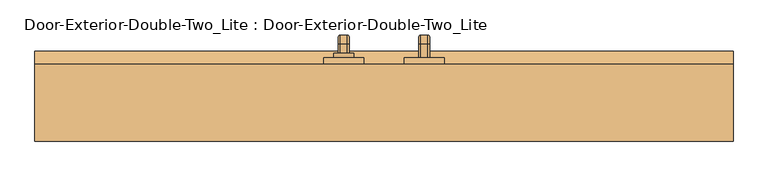
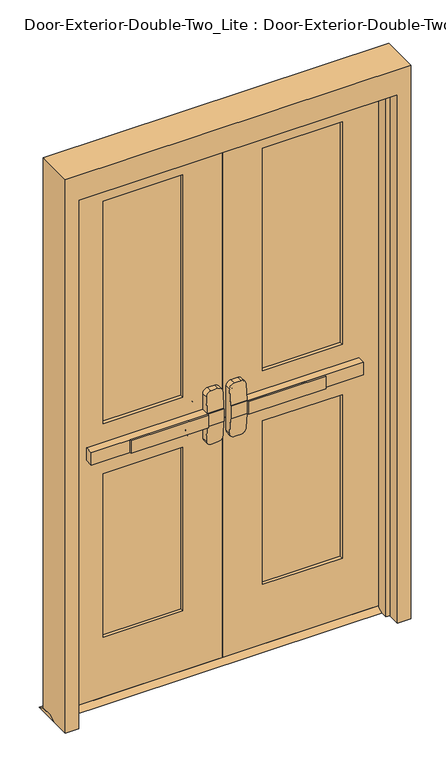
"""IFC4 building model written with IfcOpenShell, lengths in millimetres: door geometry, Door-Exterior-Double-Two_Lite : Door-Exterior-Double-Two_Lite."""

from ifc_helpers import new_model, si_unit, point, frame, frame_2d, origin, place, context, project, spatial, polyline, circle_curve, ellipse_curve, trimmed, segment, composite_curve, outline, extrude, faceted_brep, source, transform, mapped, element, save
from ifc_brep_helpers import plane_surface, cylinder_surface, revolved_surface, advanced_brep


def door_exterior_double_two_lite_door_exterior_double_two_lite_a6b01c7a(model_context):
    return source(origin(), model_context, "Body", "SolidModel", [
        extrude(outline(polyline([(-372.5333333, 12.7), (-372.5333333, 19.05), (-76.2, 19.05), (-76.2, 12.7), (-372.5333333, 12.7)])), frame((0.0, 0.0, 990.6), z_axis=(0.0, 0.0, 1.0), x_axis=(1.0, 0.0, 0.0)), (0.0, 0.0, 1.0), 50.8),
        advanced_brep(
        [(-12.7, 19.05, 1041.4), (-76.2, 19.05, 1041.4), (-520.7, 19.05, 1041.4), (-520.7, 19.05, 990.6), (-76.2, 19.05, 990.6), (-12.7, 19.05, 990.6), (-520.7, 50.8, 1041.4), (-76.2, 50.8, 1041.4), (-76.2, 50.8, 1104.9), (-57.15, 50.8, 1123.95), (-31.75, 50.8, 1123.95), (-12.7, 50.8, 1104.9), (-12.7, 50.8, 927.1), (-31.75, 50.8, 908.05), (-57.15, 50.8, 908.05), (-76.2, 50.8, 927.1), (-76.2, 50.8, 990.6), (-520.7, 50.8, 990.6), (-12.7, 22.2252467, 1041.4), (-76.2, 22.2252467, 1041.4), (-12.7, 22.2252467, 990.6), (-12.7, 27.2354269, 927.1), (-12.7, 27.2354269, 1104.9), (-76.2, 22.2252467, 990.6), (-76.2, 27.2354269, 1104.9), (-76.2, 27.2354269, 927.1), (-57.15, 28.738481, 1123.95), (-31.75, 28.738481, 1123.95), (-31.75, 28.738481, 908.05), (-57.15, 28.738481, 908.05)],
        [
            (0, 1),
            (1, 2),
            (2, 3),
            (3, 4),
            (4, 5),
            (5, 0),
            (6, 7),
            (7, 8),
            (8, 9, circle_curve(frame((-57.15, 50.8, 1104.9), z_axis=(0.0, 1.0, 0.0), x_axis=(-1.0, 0.0, 0.0)), 19.05)),
            (9, 10),
            (10, 11, circle_curve(frame((-31.75, 50.8, 1104.9), z_axis=(0.0, 1.0, 0.0), x_axis=(-1.0, 0.0, 0.0)), 19.05)),
            (11, 12),
            (12, 13, circle_curve(frame((-31.75, 50.8, 927.1), z_axis=(0.0, 1.0, 0.0), x_axis=(-1.0, 0.0, 0.0)), 19.05)),
            (13, 14),
            (14, 15, circle_curve(frame((-57.15, 50.8, 927.1), z_axis=(0.0, 1.0, 0.0), x_axis=(-1.0, 0.0, 0.0)), 19.05)),
            (15, 16),
            (16, 17),
            (17, 6),
            (0, 18),
            (18, 19),
            (19, 7),
            (6, 2),
            (5, 20),
            (20, 21),
            (21, 12),
            (11, 22),
            (22, 18),
            (16, 23),
            (23, 20),
            (3, 17),
            (19, 24),
            (24, 8),
            (15, 25),
            (25, 23),
            (9, 26),
            (26, 27),
            (27, 10),
            (13, 28),
            (28, 29),
            (29, 14),
            (29, 25, ellipse_curve(frame((-57.15, 27.2354269, 927.1), z_axis=(0.0, 0.9969018152893365, 0.07865602756830282), x_axis=(0.0, -0.07865602756830208, 0.9969018152893365)), 19.1092038, 19.05)),
            (24, 26, ellipse_curve(frame((-57.15, 27.2354269, 1104.9), z_axis=(0.0, 0.9969018152893376, -0.07865602756828934), x_axis=(0.0, -0.078656027568288, -0.9969018152893377)), 19.1092038, 19.05)),
            (27, 22, ellipse_curve(frame((-31.75, 27.2354269, 1104.9), z_axis=(0.0, 0.9969018152893376, -0.07865602756828934), x_axis=(0.0, -0.078656027568288, -0.9969018152893377)), 19.1092038, 19.05)),
            (21, 28, ellipse_curve(frame((-31.75, 27.2354269, 927.1), z_axis=(0.0, 0.9969018152893365, 0.07865602756830282), x_axis=(0.0, -0.07865602756830208, 0.9969018152893365)), 19.1092038, 19.05)),
        ],
        [
            plane_surface(frame((-12.7, 19.05, 1041.4), z_axis=(0.0, -1.0, 0.0), x_axis=(1.0, 0.0, 0.0))),
            plane_surface(frame((-12.7, 50.8, 1041.4), z_axis=(0.0, 1.0, 0.0), x_axis=(-1.0, 0.0, 0.0))),
            plane_surface(frame((-520.7, 19.05, 1041.4), z_axis=(0.0, 0.0, 1.0), x_axis=(0.0, 1.0, 0.0))),
            plane_surface(frame((-12.7, 19.05, 1041.4), z_axis=(1.0, 0.0, 0.0), x_axis=(0.0, 1.0, 0.0))),
            plane_surface(frame((-12.7, 19.05, 990.6), z_axis=(0.0, 0.0, -1.0), x_axis=(0.0, 1.0, 0.0))),
            plane_surface(frame((-520.7, 19.05, 990.6), z_axis=(-1.0, 0.0, 0.0), x_axis=(0.0, 1.0, 0.0))),
            plane_surface(frame((-76.2, 22.2252467, 927.1), z_axis=(-1.0, 0.0, 0.0), x_axis=(0.0, 1.0, 0.0))),
            plane_surface(frame((-57.15, 22.2252467, 1123.95), z_axis=(0.0, 0.0, 1.0), x_axis=(0.0, 1.0, 0.0))),
            plane_surface(frame((-31.75, 22.2252467, 908.05), z_axis=(0.0, 0.0, -1.0), x_axis=(0.0, 1.0, 0.0))),
            cylinder_surface(frame((-57.15, 50.8, 927.1), z_axis=(0.0, -1.0, 0.0), x_axis=(-1.0, 0.0, 0.0)), 19.05),
            cylinder_surface(frame((-57.15, 50.8, 1104.9), z_axis=(0.0, -1.0, 0.0), x_axis=(-1.0, 0.0, 0.0)), 19.05),
            cylinder_surface(frame((-31.75, 50.8, 1104.9), z_axis=(0.0, -1.0, 0.0), x_axis=(-1.0, 0.0, 0.0)), 19.05),
            cylinder_surface(frame((-31.75, 50.8, 927.1), z_axis=(0.0, -1.0, 0.0), x_axis=(-1.0, 0.0, 0.0)), 19.05),
            plane_surface(frame((-76.2, 22.2252467, 1041.4), z_axis=(0.0, -0.9969018152893376, 0.07865602756828934), x_axis=(1.0, 0.0, 0.0))),
            plane_surface(frame((-76.2, 28.738481, 908.05), z_axis=(0.0, -0.9969018152893365, -0.07865602756830282), x_axis=(1.0, 0.0, 0.0))),
        ],
        [
            (0, [[1, 2, 3, 4, 5, 6]]),
            (1, [[7, 8, 9, 10, 11, 12, 13, 14, 15, 16, 17, 18]]),
            (2, [[-2, -1, 19, 20, 21, -7, 22]]),
            (3, [[23, 24, 25, -12, 26, 27, -19, -6]]),
            (4, [[-17, 28, 29, -23, -5, -4, 30]]),
            (5, [[-22, -18, -30, -3]]),
            (6, [[-21, 31, 32, -8]]),
            (6, [[33, 34, -28, -16]]),
            (7, [[35, 36, 37, -10]]),
            (8, [[38, 39, 40, -14]]),
            (9, [[-40, 41, -33, -15]]),
            (10, [[-32, 42, -35, -9]]),
            (11, [[-37, 43, -26, -11]]),
            (12, [[-25, 44, -38, -13]]),
            (13, [[-27, -43, -36, -42, -31, -20]]),
            (14, [[-29, -34, -41, -39, -44, -24]]),
        ],
    ),
        extrude(outline(polyline([(95.25, 12.7), (120.65, 0.0), (25.4, 0.0), (50.8, 12.7), (95.25, 12.7)])), frame((-660.4, 0.0, 0.0), z_axis=(1.0, 0.0, 0.0), x_axis=(0.0, 1.0, 0.0)), (0.0, 0.0, 1.0), 1320.8),
        extrude(outline(polyline([(372.5333333, 12.7), (76.2, 12.7), (76.2, 19.05), (372.5333333, 19.05), (372.5333333, 12.7)])), frame((0.0, 0.0, 990.6), z_axis=(0.0, 0.0, 1.0), x_axis=(1.0, 0.0, 0.0)), (0.0, 0.0, 1.0), 50.8),
        advanced_brep(
        [(12.7, 19.05, 1041.4), (12.7, 19.05, 990.6), (76.2, 19.05, 990.6), (520.7, 19.05, 990.6), (520.7, 19.05, 1041.4), (76.2, 19.05, 1041.4), (520.7, 50.8, 1041.4), (520.7, 50.8, 990.6), (76.2, 50.8, 990.6), (76.2, 50.8, 927.1), (57.15, 50.8, 908.05), (31.75, 50.8, 908.05), (12.7, 50.8, 927.1), (12.7, 50.8, 1104.9), (31.75, 50.8, 1123.95), (57.15, 50.8, 1123.95), (76.2, 50.8, 1104.9), (76.2, 50.8, 1041.4), (76.2, 22.2252467, 1041.4), (12.7, 22.2252467, 1041.4), (12.7, 27.2354269, 1104.9), (12.7, 27.2354269, 927.1), (12.7, 22.2252467, 990.6), (76.2, 22.2252467, 990.6), (76.2, 27.2354269, 927.1), (76.2, 27.2354269, 1104.9), (31.75, 28.738481, 1123.95), (57.15, 28.738481, 1123.95), (57.15, 28.738481, 908.05), (31.75, 28.738481, 908.05)],
        [
            (0, 1),
            (1, 2),
            (2, 3),
            (3, 4),
            (4, 5),
            (5, 0),
            (6, 7),
            (7, 8),
            (8, 9),
            (9, 10, circle_curve(frame((57.15, 50.8, 927.1), z_axis=(0.0, 1.0, 0.0), x_axis=(1.0, 0.0, 0.0)), 19.05)),
            (10, 11),
            (11, 12, circle_curve(frame((31.75, 50.8, 927.1), z_axis=(0.0, 1.0, 0.0), x_axis=(1.0, 0.0, 0.0)), 19.05)),
            (12, 13),
            (13, 14, circle_curve(frame((31.75, 50.8, 1104.9), z_axis=(0.0, 1.0, 0.0), x_axis=(1.0, 0.0, 0.0)), 19.05)),
            (14, 15),
            (15, 16, circle_curve(frame((57.15, 50.8, 1104.9), z_axis=(0.0, 1.0, 0.0), x_axis=(1.0, 0.0, 0.0)), 19.05)),
            (16, 17),
            (17, 6),
            (4, 6),
            (17, 18),
            (18, 19),
            (19, 0),
            (19, 20),
            (20, 13),
            (12, 21),
            (21, 22),
            (22, 1),
            (7, 3),
            (22, 23),
            (23, 8),
            (23, 24),
            (24, 9),
            (16, 25),
            (25, 18),
            (14, 26),
            (26, 27),
            (27, 15),
            (10, 28),
            (28, 29),
            (29, 11),
            (24, 28, ellipse_curve(frame((57.15, 27.2354269, 927.1), z_axis=(0.0, 0.9969018152893365, 0.07865602756830282), x_axis=(0.0, -0.07865602756830208, 0.9969018152893365)), 19.1092038, 19.05)),
            (27, 25, ellipse_curve(frame((57.15, 27.2354269, 1104.9), z_axis=(0.0, 0.9969018152893376, -0.07865602756828934), x_axis=(0.0, -0.078656027568288, -0.9969018152893377)), 19.1092038, 19.05)),
            (20, 26, ellipse_curve(frame((31.75, 27.2354269, 1104.9), z_axis=(0.0, 0.9969018152893376, -0.07865602756828934), x_axis=(0.0, -0.078656027568288, -0.9969018152893377)), 19.1092038, 19.05)),
            (29, 21, ellipse_curve(frame((31.75, 27.2354269, 927.1), z_axis=(0.0, 0.9969018152893365, 0.07865602756830282), x_axis=(0.0, -0.07865602756830208, 0.9969018152893365)), 19.1092038, 19.05)),
        ],
        [
            plane_surface(frame((12.7, 19.05, 1041.4), z_axis=(0.0, -1.0, 0.0), x_axis=(-1.0, 0.0, 0.0))),
            plane_surface(frame((12.7, 50.8, 1041.4), z_axis=(0.0, 1.0, 0.0), x_axis=(1.0, 0.0, 0.0))),
            plane_surface(frame((520.7, 19.05, 1041.4), z_axis=(0.0, 0.0, 1.0), x_axis=(0.0, 1.0, 0.0))),
            plane_surface(frame((12.7, 19.05, 1041.4), z_axis=(-1.0, 0.0, 0.0), x_axis=(0.0, 1.0, 0.0))),
            plane_surface(frame((12.7, 19.05, 990.6), z_axis=(0.0, 0.0, -1.0), x_axis=(0.0, 1.0, 0.0))),
            plane_surface(frame((520.7, 19.05, 990.6), z_axis=(1.0, 0.0, 0.0), x_axis=(0.0, 1.0, 0.0))),
            plane_surface(frame((76.2, 22.2252467, 927.1), z_axis=(1.0, 0.0, 0.0), x_axis=(0.0, 1.0, 0.0))),
            plane_surface(frame((57.15, 22.2252467, 1123.95), z_axis=(0.0, 0.0, 1.0), x_axis=(0.0, 1.0, 0.0))),
            plane_surface(frame((31.75, 22.2252467, 908.05), z_axis=(0.0, 0.0, -1.0), x_axis=(0.0, 1.0, 0.0))),
            cylinder_surface(frame((57.15, 50.8, 927.1), z_axis=(0.0, -1.0, 0.0), x_axis=(1.0, 0.0, 0.0)), 19.05),
            cylinder_surface(frame((57.15, 50.8, 1104.9), z_axis=(0.0, -1.0, 0.0), x_axis=(1.0, 0.0, 0.0)), 19.05),
            cylinder_surface(frame((31.75, 50.8, 1104.9), z_axis=(0.0, -1.0, 0.0), x_axis=(1.0, 0.0, 0.0)), 19.05),
            cylinder_surface(frame((31.75, 50.8, 927.1), z_axis=(0.0, -1.0, 0.0), x_axis=(1.0, 0.0, 0.0)), 19.05),
            plane_surface(frame((76.2, 22.2252467, 1041.4), z_axis=(0.0, -0.9969018152893376, 0.07865602756828934), x_axis=(-1.0, 0.0, 0.0))),
            plane_surface(frame((76.2, 28.738481, 908.05), z_axis=(0.0, -0.9969018152893365, -0.07865602756830282), x_axis=(-1.0, 0.0, 0.0))),
        ],
        [
            (0, [[1, 2, 3, 4, 5, 6]]),
            (1, [[7, 8, 9, 10, 11, 12, 13, 14, 15, 16, 17, 18]]),
            (2, [[19, -18, 20, 21, 22, -6, -5]]),
            (3, [[-1, -22, 23, 24, -13, 25, 26, 27]]),
            (4, [[28, -3, -2, -27, 29, 30, -8]]),
            (5, [[-4, -28, -7, -19]]),
            (6, [[-9, -30, 31, 32]]),
            (6, [[-17, 33, 34, -20]]),
            (7, [[-15, 35, 36, 37]]),
            (8, [[-11, 38, 39, 40]]),
            (9, [[-10, -32, 41, -38]]),
            (10, [[-16, -37, 42, -33]]),
            (11, [[-14, -24, 43, -35]]),
            (12, [[-12, -40, 44, -25]]),
            (13, [[-21, -34, -42, -36, -43, -23]]),
            (14, [[-26, -44, -39, -41, -31, -29]]),
        ],
    ),
        advanced_brep(
        [(66.2, 107.95, 1017.190625), (66.2, 107.95, 1014.809375), (69.771875, 107.95, 1011.2375), (82.6284594, 107.95, 1011.2375), (86.2, 107.95, 1014.8090406), (86.2, 107.95, 1017.190625), (82.628125, 107.95, 1020.7625), (69.771875, 107.95, 1020.7625), (66.2, 107.95, 887.809375), (69.771875, 107.95, 884.2375), (82.628125, 107.95, 884.2375), (86.2, 107.95, 887.809375), (86.2, 107.95, 890.1909594), (82.6284594, 107.95, 893.7625), (69.771875, 107.95, 893.7625), (66.2, 107.95, 890.190625), (66.2, 133.35, 1017.190625), (66.2, 147.240625, 1003.3), (66.2, 147.240625, 901.7), (66.2, 133.35, 887.809375), (66.2, 133.35, 890.190625), (66.2, 144.859375, 901.7), (66.2, 144.859375, 1003.3), (66.2, 133.35, 1014.809375), (69.771875, 133.35, 1011.2375), (82.6284594, 133.35, 1011.2375), (86.2, 133.35, 1014.8090406), (86.2, 144.8590406, 1003.3), (86.2, 144.8590406, 901.7), (86.2, 133.35, 890.1909594), (86.2, 133.35, 887.809375), (86.2, 147.240625, 901.7), (86.2, 147.240625, 1003.3), (86.2, 133.35, 1017.190625), (82.628125, 133.35, 1020.7625), (69.771875, 133.35, 1020.7625), (69.771875, 141.2875, 1003.3), (82.6284594, 141.2875, 1003.3), (82.628125, 150.8125, 1003.3), (69.771875, 150.8125, 1003.3), (69.771875, 141.2875, 901.7), (82.6284594, 141.2875, 901.7), (82.628125, 150.8125, 901.7), (69.771875, 150.8125, 901.7), (69.771875, 133.35, 893.7625), (82.6284594, 133.35, 893.7625), (82.628125, 133.35, 884.2375), (69.771875, 133.35, 884.2375)],
        [
            (0, 1),
            (1, 2, circle_curve(frame((69.771875, 107.95, 1014.809375), z_axis=(0.0, -1.0, 0.0), x_axis=(0.0, 0.0, 1.0)), 3.571875)),
            (2, 3),
            (3, 4, circle_curve(frame((82.6284594, 107.95, 1014.8090406), z_axis=(0.0, -1.0, 0.0), x_axis=(0.0, 0.0, 1.0)), 3.5715406)),
            (4, 5),
            (5, 6, circle_curve(frame((82.628125, 107.95, 1017.190625), z_axis=(0.0, -1.0, 0.0), x_axis=(0.0, 0.0, 1.0)), 3.571875)),
            (6, 7),
            (7, 0, circle_curve(frame((69.771875, 107.95, 1017.190625), z_axis=(0.0, -1.0, 0.0), x_axis=(0.0, 0.0, 1.0)), 3.571875)),
            (8, 9, circle_curve(frame((69.771875, 107.95, 887.809375), z_axis=(0.0, -1.0, 0.0), x_axis=(0.0, 0.0, -1.0)), 3.571875)),
            (9, 10),
            (10, 11, circle_curve(frame((82.628125, 107.95, 887.809375), z_axis=(0.0, -1.0, 0.0), x_axis=(0.0, 0.0, -1.0)), 3.571875)),
            (11, 12),
            (12, 13, circle_curve(frame((82.6284594, 107.95, 890.1909594), z_axis=(0.0, -1.0, 0.0), x_axis=(0.0, 0.0, -1.0)), 3.5715406)),
            (13, 14),
            (14, 15, circle_curve(frame((69.771875, 107.95, 890.190625), z_axis=(0.0, -1.0, 0.0), x_axis=(0.0, 0.0, -1.0)), 3.571875)),
            (15, 8),
            (0, 16),
            (16, 17, circle_curve(frame((66.2, 133.35, 1003.3), z_axis=(-1.0, 0.0, 0.0), x_axis=(0.0, 0.0, 1.0)), 13.890625)),
            (17, 18),
            (18, 19, circle_curve(frame((66.2, 133.35, 901.7), z_axis=(-1.0, 0.0, 0.0), x_axis=(0.0, 1.0, 0.0)), 13.890625)),
            (19, 8),
            (15, 20),
            (20, 21, circle_curve(frame((66.2, 133.35, 901.7), z_axis=(1.0, 0.0, 0.0), x_axis=(0.0, 1.0, 0.0)), 11.509375)),
            (21, 22),
            (22, 23, circle_curve(frame((66.2, 133.35, 1003.3), z_axis=(1.0, 0.0, 0.0), x_axis=(0.0, 0.0, 1.0)), 11.509375)),
            (23, 1),
            (23, 24, circle_curve(frame((69.771875, 133.35, 1014.809375), z_axis=(0.0, -1.0, 0.0), x_axis=(0.0, 0.0, 1.0)), 3.571875)),
            (24, 2),
            (24, 25),
            (25, 3),
            (25, 26, circle_curve(frame((82.6284594, 133.35, 1014.8090406), z_axis=(0.0, -1.0, 0.0), x_axis=(0.0, 0.0, 1.0)), 3.5715406)),
            (26, 4),
            (26, 27, circle_curve(frame((86.2, 133.35, 1003.3), z_axis=(-1.0, 0.0, 0.0), x_axis=(0.0, 0.0, 1.0)), 11.5090406)),
            (27, 28),
            (28, 29, circle_curve(frame((86.2, 133.35, 901.7), z_axis=(-1.0, 0.0, 0.0), x_axis=(0.0, 1.0, 0.0)), 11.5090406)),
            (29, 12),
            (11, 30),
            (30, 31, circle_curve(frame((86.2, 133.35, 901.7), z_axis=(1.0, 0.0, 0.0), x_axis=(0.0, 1.0, 0.0)), 13.890625)),
            (31, 32),
            (32, 33, circle_curve(frame((86.2, 133.35, 1003.3), z_axis=(1.0, 0.0, 0.0), x_axis=(0.0, 0.0, 1.0)), 13.890625)),
            (33, 5),
            (33, 34, circle_curve(frame((82.628125, 133.35, 1017.190625), z_axis=(0.0, -1.0, 0.0), x_axis=(0.0, 0.0, 1.0)), 3.571875)),
            (34, 6),
            (34, 35),
            (35, 7),
            (35, 16, circle_curve(frame((69.771875, 133.35, 1017.190625), z_axis=(0.0, -1.0, 0.0), x_axis=(0.0, 0.0, 1.0)), 3.571875)),
            (36, 24, circle_curve(frame((69.771875, 133.35, 1003.3), z_axis=(1.0, 0.0, 0.0), x_axis=(0.0, 0.0, 1.0)), 7.9375)),
            (22, 36, circle_curve(frame((69.771875, 144.859375, 1003.3), z_axis=(0.0, 0.0, 1.0), x_axis=(0.0, 1.0, 0.0)), 3.571875)),
            (37, 25, circle_curve(frame((82.6284594, 133.35, 1003.3), z_axis=(1.0, 0.0, 0.0), x_axis=(0.0, 0.0, 1.0)), 7.9375)),
            (36, 37),
            (37, 27, circle_curve(frame((82.6284594, 144.8590406, 1003.3), z_axis=(0.0, 0.0, 1.0), x_axis=(0.0, 1.0, 0.0)), 3.5715406)),
            (38, 34, circle_curve(frame((82.628125, 133.35, 1003.3), z_axis=(1.0, 0.0, 0.0), x_axis=(0.0, 0.0, 1.0)), 17.4625)),
            (32, 38, circle_curve(frame((82.628125, 147.240625, 1003.3), z_axis=(0.0, 0.0, 1.0), x_axis=(0.0, 1.0, 0.0)), 3.571875)),
            (39, 35, circle_curve(frame((69.771875, 133.35, 1003.3), z_axis=(1.0, 0.0, 0.0), x_axis=(0.0, 0.0, 1.0)), 17.4625)),
            (38, 39),
            (39, 17, circle_curve(frame((69.771875, 147.240625, 1003.3), z_axis=(0.0, 0.0, 1.0), x_axis=(0.0, 1.0, 0.0)), 3.571875)),
            (21, 40, circle_curve(frame((69.771875, 144.859375, 901.7), z_axis=(0.0, 0.0, 1.0), x_axis=(0.0, 1.0, 0.0)), 3.571875)),
            (40, 36),
            (40, 41),
            (41, 37),
            (41, 28, circle_curve(frame((82.6284594, 144.8590406, 901.7), z_axis=(0.0, 0.0, 1.0), x_axis=(0.0, 1.0, 0.0)), 3.5715406)),
            (31, 42, circle_curve(frame((82.628125, 147.240625, 901.7), z_axis=(0.0, 0.0, 1.0), x_axis=(0.0, 1.0, 0.0)), 3.571875)),
            (42, 38),
            (42, 43),
            (43, 39),
            (43, 18, circle_curve(frame((69.771875, 147.240625, 901.7), z_axis=(0.0, 0.0, 1.0), x_axis=(0.0, 1.0, 0.0)), 3.571875)),
            (44, 40, circle_curve(frame((69.771875, 133.35, 901.7), z_axis=(1.0, 0.0, 0.0), x_axis=(0.0, 1.0, 0.0)), 7.9375)),
            (20, 44, circle_curve(frame((69.771875, 133.35, 890.190625), z_axis=(0.0, 1.0, 0.0), x_axis=(0.0, 0.0, -1.0)), 3.571875)),
            (45, 41, circle_curve(frame((82.6284594, 133.35, 901.7), z_axis=(1.0, 0.0, 0.0), x_axis=(0.0, 1.0, 0.0)), 7.9375)),
            (44, 45),
            (45, 29, circle_curve(frame((82.6284594, 133.35, 890.1909594), z_axis=(0.0, 1.0, 0.0), x_axis=(0.0, 0.0, -1.0)), 3.5715406)),
            (46, 42, circle_curve(frame((82.628125, 133.35, 901.7), z_axis=(1.0, 0.0, 0.0), x_axis=(0.0, 1.0, 0.0)), 17.4625)),
            (30, 46, circle_curve(frame((82.628125, 133.35, 887.809375), z_axis=(0.0, 1.0, 0.0), x_axis=(0.0, 0.0, -1.0)), 3.571875)),
            (47, 43, circle_curve(frame((69.771875, 133.35, 901.7), z_axis=(1.0, 0.0, 0.0), x_axis=(0.0, 1.0, 0.0)), 17.4625)),
            (46, 47),
            (47, 19, circle_curve(frame((69.771875, 133.35, 887.809375), z_axis=(0.0, 1.0, 0.0), x_axis=(0.0, 0.0, -1.0)), 3.571875)),
            (14, 44),
            (13, 45),
            (10, 46),
            (9, 47),
        ],
        [
            plane_surface(frame((76.2, 107.95, 1016.0), z_axis=(0.0, -1.0, 0.0), x_axis=(1.0, 0.0, 0.0))),
            plane_surface(frame((76.2, 107.95, 889.0), z_axis=(0.0, -1.0, 0.0), x_axis=(1.0, 0.0, 0.0))),
            plane_surface(frame((66.2, 107.95, 1017.190625), z_axis=(-1.0, 0.0, 0.0), x_axis=(0.0, 1.0, 0.0))),
            cylinder_surface(frame((69.771875, 107.95, 1014.809375), z_axis=(0.0, -1.0, 0.0), x_axis=(0.0, 0.0, 1.0)), 3.571875),
            plane_surface(frame((69.771875, 107.95, 1011.2375), z_axis=(0.0, 0.0, -1.0), x_axis=(0.0, 1.0, 0.0))),
            cylinder_surface(frame((82.6284594, 107.95, 1014.8090406), z_axis=(0.0, -1.0, 0.0), x_axis=(0.0, 0.0, 1.0)), 3.5715406),
            plane_surface(frame((86.2, 107.95, 1014.8090406), z_axis=(1.0, 0.0, 0.0), x_axis=(0.0, 1.0, 0.0))),
            cylinder_surface(frame((82.628125, 107.95, 1017.190625), z_axis=(0.0, -1.0, 0.0), x_axis=(0.0, 0.0, 1.0)), 3.571875),
            plane_surface(frame((82.628125, 107.95, 1020.7625), z_axis=(0.0, 0.0, 1.0), x_axis=(0.0, 1.0, 0.0))),
            cylinder_surface(frame((69.771875, 107.95, 1017.190625), z_axis=(0.0, -1.0, 0.0), x_axis=(0.0, 0.0, 1.0)), 3.571875),
            revolved_surface(trimmed(ellipse_curve(frame((69.771875, 133.35, 1014.809375), z_axis=(0.0, -1.0, 0.0), x_axis=(0.0, 0.0, 1.0)), 3.571875, 3.571875), [point((66.2, 133.35, 1014.809375))], [point((69.771875, 133.35, 1011.2375))], True, "CARTESIAN"), (76.2, 133.35, 1003.3), (-1.0, 0.0, 0.0)),
            revolved_surface(polyline([(69.771875, 133.35, 1011.2375), (82.6284594, 133.35, 1011.2375)]), (76.2, 133.35, 1003.3), (-1.0, 0.0, 0.0)),
            revolved_surface(trimmed(ellipse_curve(frame((82.6284594, 133.35, 1014.8090406), z_axis=(0.0, -1.0, 0.0), x_axis=(0.0, 0.0, 1.0)), 3.5715406, 3.5715406), [point((82.6284594, 133.35, 1011.2375))], [point((86.2, 133.35, 1014.8090406))], True, "CARTESIAN"), (76.2, 133.35, 1003.3), (-1.0, 0.0, 0.0)),
            revolved_surface(trimmed(ellipse_curve(frame((82.628125, 133.35, 1017.190625), z_axis=(0.0, -1.0, 0.0), x_axis=(0.0, 0.0, 1.0)), 3.571875, 3.571875), [point((86.2, 133.35, 1017.190625))], [point((82.628125, 133.35, 1020.7625))], True, "CARTESIAN"), (76.2, 133.35, 1003.3), (-1.0, 0.0, 0.0)),
            cylinder_surface(frame((76.2, 133.35, 1003.3), z_axis=(-1.0, 0.0, 0.0), x_axis=(0.0, 0.0, 1.0)), 17.4625),
            revolved_surface(trimmed(ellipse_curve(frame((69.771875, 133.35, 1017.190625), z_axis=(0.0, -1.0, 0.0), x_axis=(0.0, 0.0, 1.0)), 3.571875, 3.571875), [point((69.771875, 133.35, 1020.7625))], [point((66.2, 133.35, 1017.190625))], True, "CARTESIAN"), (76.2, 133.35, 1003.3), (-1.0, 0.0, 0.0)),
            cylinder_surface(frame((69.771875, 144.859375, 1003.3), z_axis=(0.0, 0.0, 1.0), x_axis=(0.0, 1.0, 0.0)), 3.571875),
            plane_surface(frame((69.771875, 141.2875, 1003.3), z_axis=(0.0, -1.0, 0.0), x_axis=(0.0, 0.0, -1.0))),
            cylinder_surface(frame((82.6284594, 144.8590406, 1003.3), z_axis=(0.0, 0.0, 1.0), x_axis=(0.0, 1.0, 0.0)), 3.5715406),
            cylinder_surface(frame((82.628125, 147.240625, 1003.3), z_axis=(0.0, 0.0, 1.0), x_axis=(0.0, 1.0, 0.0)), 3.571875),
            plane_surface(frame((82.628125, 150.8125, 1003.3), z_axis=(0.0, 1.0, 0.0), x_axis=(0.0, 0.0, -1.0))),
            cylinder_surface(frame((69.771875, 147.240625, 1003.3), z_axis=(0.0, 0.0, 1.0), x_axis=(0.0, 1.0, 0.0)), 3.571875),
            revolved_surface(trimmed(ellipse_curve(frame((69.771875, 144.859375, 901.7), z_axis=(0.0, 0.0, 1.0), x_axis=(0.0, 1.0, 0.0)), 3.571875, 3.571875), [point((66.2, 144.859375, 901.7))], [point((69.771875, 141.2875, 901.7))], True, "CARTESIAN"), (76.2, 133.35, 901.7), (-1.0, 0.0, 0.0)),
            revolved_surface(polyline([(69.771875, 141.2875, 901.7), (82.6284594, 141.2875, 901.7)]), (76.2, 133.35, 901.7), (-1.0, 0.0, 0.0)),
            revolved_surface(trimmed(ellipse_curve(frame((82.6284594, 144.8590406, 901.7), z_axis=(0.0, 0.0, 1.0), x_axis=(0.0, 1.0, 0.0)), 3.5715406, 3.5715406), [point((82.6284594, 141.2875, 901.7))], [point((86.2, 144.8590406, 901.7))], True, "CARTESIAN"), (76.2, 133.35, 901.7), (-1.0, 0.0, 0.0)),
            revolved_surface(trimmed(ellipse_curve(frame((82.628125, 147.240625, 901.7), z_axis=(0.0, 0.0, 1.0), x_axis=(0.0, 1.0, 0.0)), 3.571875, 3.571875), [point((86.2, 147.240625, 901.7))], [point((82.628125, 150.8125, 901.7))], True, "CARTESIAN"), (76.2, 133.35, 901.7), (-1.0, 0.0, 0.0)),
            cylinder_surface(frame((76.2, 133.35, 901.7), z_axis=(-1.0, 0.0, 0.0), x_axis=(0.0, 1.0, 0.0)), 17.4625),
            revolved_surface(trimmed(ellipse_curve(frame((69.771875, 147.240625, 901.7), z_axis=(0.0, 0.0, 1.0), x_axis=(0.0, 1.0, 0.0)), 3.571875, 3.571875), [point((69.771875, 150.8125, 901.7))], [point((66.2, 147.240625, 901.7))], True, "CARTESIAN"), (76.2, 133.35, 901.7), (-1.0, 0.0, 0.0)),
            cylinder_surface(frame((69.771875, 133.35, 890.190625), z_axis=(0.0, 1.0, 0.0), x_axis=(0.0, 0.0, -1.0)), 3.571875),
            plane_surface(frame((69.771875, 133.35, 893.7625), z_axis=(0.0, 0.0, 1.0), x_axis=(0.0, -1.0, 0.0))),
            cylinder_surface(frame((82.6284594, 133.35, 890.1909594), z_axis=(0.0, 1.0, 0.0), x_axis=(0.0, 0.0, -1.0)), 3.5715406),
            cylinder_surface(frame((82.628125, 133.35, 887.809375), z_axis=(0.0, 1.0, 0.0), x_axis=(0.0, 0.0, -1.0)), 3.571875),
            plane_surface(frame((82.628125, 133.35, 884.2375), z_axis=(0.0, 0.0, -1.0), x_axis=(0.0, -1.0, 0.0))),
            cylinder_surface(frame((69.771875, 133.35, 887.809375), z_axis=(0.0, 1.0, 0.0), x_axis=(0.0, 0.0, -1.0)), 3.571875),
        ],
        [
            (0, [[1, 2, 3, 4, 5, 6, 7, 8]]),
            (1, [[9, 10, 11, 12, 13, 14, 15, 16]]),
            (2, [[-1, 17, 18, 19, 20, 21, -16, 22, 23, 24, 25, 26]]),
            (3, [[-2, -26, 27, 28]]),
            (4, [[-3, -28, 29, 30]]),
            (5, [[-4, -30, 31, 32]]),
            (6, [[-5, -32, 33, 34, 35, 36, -12, 37, 38, 39, 40, 41]]),
            (7, [[-6, -41, 42, 43]]),
            (8, [[-7, -43, 44, 45]]),
            (9, [[-8, -45, 46, -17]]),
            (10, [[47, -27, -25, 48]]),
            (11, [[49, -29, -47, 50]]),
            (12, [[-33, -31, -49, 51]]),
            (13, [[52, -42, -40, 53]]),
            (14, [[54, -44, -52, 55]]),
            (15, [[-18, -46, -54, 56]]),
            (16, [[-48, -24, 57, 58]]),
            (17, [[-50, -58, 59, 60]]),
            (18, [[-51, -60, 61, -34]]),
            (19, [[-53, -39, 62, 63]]),
            (20, [[-55, -63, 64, 65]]),
            (21, [[-56, -65, 66, -19]]),
            (22, [[67, -57, -23, 68]]),
            (23, [[69, -59, -67, 70]]),
            (24, [[-35, -61, -69, 71]]),
            (25, [[72, -62, -38, 73]]),
            (26, [[74, -64, -72, 75]]),
            (27, [[-20, -66, -74, 76]]),
            (28, [[-68, -22, -15, 77]]),
            (29, [[-70, -77, -14, 78]]),
            (30, [[-71, -78, -13, -36]]),
            (31, [[-73, -37, -11, 79]]),
            (32, [[-75, -79, -10, 80]]),
            (33, [[-76, -80, -9, -21]]),
        ],
    ),
        extrude(outline(composite_curve([segment(trimmed(circle_curve(frame_2d((1113.0338574, 76.2)), 89.3016225), [point((1193.8, 114.3))], [point((1193.8, 38.1))], False, "CARTESIAN"), True, "CONTINUOUS"), segment(polyline([(1193.8, 38.1), (838.2, 38.1)]), True, "CONTINUOUS"), segment(trimmed(circle_curve(frame_2d((918.9661426, 76.2)), 89.3016225), [point((838.2, 38.1))], [point((838.2, 114.3))], False, "CARTESIAN"), True, "CONTINUOUS"), segment(polyline([(838.2, 114.3), (1193.8, 114.3)]), True, "CONTINUOUS")], self_intersect=False)), frame((0.0, 95.25, 0.0), z_axis=(0.0, 1.0, 0.0), x_axis=(0.0, 0.0, 1.0)), (0.0, 0.0, 1.0), 12.7),
        advanced_brep(
        [(-86.2, 107.95, 1017.190625), (-86.2, 107.95, 1014.809375), (-82.628125, 107.95, 1011.2375), (-69.7715406, 107.95, 1011.2375), (-66.2, 107.95, 1014.8090406), (-66.2, 107.95, 1017.190625), (-69.771875, 107.95, 1020.7625), (-82.628125, 107.95, 1020.7625), (-86.2, 107.95, 887.809375), (-82.628125, 107.95, 884.2375), (-69.771875, 107.95, 884.2375), (-66.2, 107.95, 887.809375), (-66.2, 107.95, 890.1909594), (-69.7715406, 107.95, 893.7625), (-82.628125, 107.95, 893.7625), (-86.2, 107.95, 890.190625), (-86.2, 133.35, 1017.190625), (-86.2, 147.240625, 1003.3), (-86.2, 147.240625, 901.7), (-86.2, 133.35, 887.809375), (-86.2, 133.35, 890.190625), (-86.2, 144.859375, 901.7), (-86.2, 144.859375, 1003.3), (-86.2, 133.35, 1014.809375), (-82.628125, 133.35, 1011.2375), (-69.7715406, 133.35, 1011.2375), (-66.2, 133.35, 1014.8090406), (-66.2, 144.8590406, 1003.3), (-66.2, 144.8590406, 901.7), (-66.2, 133.35, 890.1909594), (-66.2, 133.35, 887.809375), (-66.2, 147.240625, 901.7), (-66.2, 147.240625, 1003.3), (-66.2, 133.35, 1017.190625), (-69.771875, 133.35, 1020.7625), (-82.628125, 133.35, 1020.7625), (-82.628125, 141.2875, 1003.3), (-69.7715406, 141.2875, 1003.3), (-69.771875, 150.8125, 1003.3), (-82.628125, 150.8125, 1003.3), (-82.628125, 141.2875, 901.7), (-69.7715406, 141.2875, 901.7), (-69.771875, 150.8125, 901.7), (-82.628125, 150.8125, 901.7), (-82.628125, 133.35, 893.7625), (-69.7715406, 133.35, 893.7625), (-69.771875, 133.35, 884.2375), (-82.628125, 133.35, 884.2375)],
        [
            (0, 1),
            (1, 2, circle_curve(frame((-82.628125, 107.95, 1014.809375), z_axis=(0.0, -1.0, 0.0), x_axis=(0.0, 0.0, 1.0)), 3.571875)),
            (2, 3),
            (3, 4, circle_curve(frame((-69.7715406, 107.95, 1014.8090406), z_axis=(0.0, -1.0, 0.0), x_axis=(0.0, 0.0, 1.0)), 3.5715406)),
            (4, 5),
            (5, 6, circle_curve(frame((-69.771875, 107.95, 1017.190625), z_axis=(0.0, -1.0, 0.0), x_axis=(0.0, 0.0, 1.0)), 3.571875)),
            (6, 7),
            (7, 0, circle_curve(frame((-82.628125, 107.95, 1017.190625), z_axis=(0.0, -1.0, 0.0), x_axis=(0.0, 0.0, 1.0)), 3.571875)),
            (8, 9, circle_curve(frame((-82.628125, 107.95, 887.809375), z_axis=(0.0, -1.0, 0.0), x_axis=(0.0, 0.0, -1.0)), 3.571875)),
            (9, 10),
            (10, 11, circle_curve(frame((-69.771875, 107.95, 887.809375), z_axis=(0.0, -1.0, 0.0), x_axis=(0.0, 0.0, -1.0)), 3.571875)),
            (11, 12),
            (12, 13, circle_curve(frame((-69.7715406, 107.95, 890.1909594), z_axis=(0.0, -1.0, 0.0), x_axis=(0.0, 0.0, -1.0)), 3.5715406)),
            (13, 14),
            (14, 15, circle_curve(frame((-82.628125, 107.95, 890.190625), z_axis=(0.0, -1.0, 0.0), x_axis=(0.0, 0.0, -1.0)), 3.571875)),
            (15, 8),
            (0, 16),
            (16, 17, circle_curve(frame((-86.2, 133.35, 1003.3), z_axis=(-1.0, 0.0, 0.0), x_axis=(0.0, 0.0, 1.0)), 13.890625)),
            (17, 18),
            (18, 19, circle_curve(frame((-86.2, 133.35, 901.7), z_axis=(-1.0, 0.0, 0.0), x_axis=(0.0, 1.0, 0.0)), 13.890625)),
            (19, 8),
            (15, 20),
            (20, 21, circle_curve(frame((-86.2, 133.35, 901.7), z_axis=(1.0, 0.0, 0.0), x_axis=(0.0, 1.0, 0.0)), 11.509375)),
            (21, 22),
            (22, 23, circle_curve(frame((-86.2, 133.35, 1003.3), z_axis=(1.0, 0.0, 0.0), x_axis=(0.0, 0.0, 1.0)), 11.509375)),
            (23, 1),
            (23, 24, circle_curve(frame((-82.628125, 133.35, 1014.809375), z_axis=(0.0, -1.0, 0.0), x_axis=(0.0, 0.0, 1.0)), 3.571875)),
            (24, 2),
            (24, 25),
            (25, 3),
            (25, 26, circle_curve(frame((-69.7715406, 133.35, 1014.8090406), z_axis=(0.0, -1.0, 0.0), x_axis=(0.0, 0.0, 1.0)), 3.5715406)),
            (26, 4),
            (26, 27, circle_curve(frame((-66.2, 133.35, 1003.3), z_axis=(-1.0, 0.0, 0.0), x_axis=(0.0, 0.0, 1.0)), 11.5090406)),
            (27, 28),
            (28, 29, circle_curve(frame((-66.2, 133.35, 901.7), z_axis=(-1.0, 0.0, 0.0), x_axis=(0.0, 1.0, 0.0)), 11.5090406)),
            (29, 12),
            (11, 30),
            (30, 31, circle_curve(frame((-66.2, 133.35, 901.7), z_axis=(1.0, 0.0, 0.0), x_axis=(0.0, 1.0, 0.0)), 13.890625)),
            (31, 32),
            (32, 33, circle_curve(frame((-66.2, 133.35, 1003.3), z_axis=(1.0, 0.0, 0.0), x_axis=(0.0, 0.0, 1.0)), 13.890625)),
            (33, 5),
            (33, 34, circle_curve(frame((-69.771875, 133.35, 1017.190625), z_axis=(0.0, -1.0, 0.0), x_axis=(0.0, 0.0, 1.0)), 3.571875)),
            (34, 6),
            (34, 35),
            (35, 7),
            (35, 16, circle_curve(frame((-82.628125, 133.35, 1017.190625), z_axis=(0.0, -1.0, 0.0), x_axis=(0.0, 0.0, 1.0)), 3.571875)),
            (36, 24, circle_curve(frame((-82.628125, 133.35, 1003.3), z_axis=(1.0, 0.0, 0.0), x_axis=(0.0, 0.0, 1.0)), 7.9375)),
            (22, 36, circle_curve(frame((-82.628125, 144.859375, 1003.3), z_axis=(0.0, 0.0, 1.0), x_axis=(0.0, 1.0, 0.0)), 3.571875)),
            (37, 25, circle_curve(frame((-69.7715406, 133.35, 1003.3), z_axis=(1.0, 0.0, 0.0), x_axis=(0.0, 0.0, 1.0)), 7.9375)),
            (36, 37),
            (37, 27, circle_curve(frame((-69.7715406, 144.8590406, 1003.3), z_axis=(0.0, 0.0, 1.0), x_axis=(0.0, 1.0, 0.0)), 3.5715406)),
            (38, 34, circle_curve(frame((-69.771875, 133.35, 1003.3), z_axis=(1.0, 0.0, 0.0), x_axis=(0.0, 0.0, 1.0)), 17.4625)),
            (32, 38, circle_curve(frame((-69.771875, 147.240625, 1003.3), z_axis=(0.0, 0.0, 1.0), x_axis=(0.0, 1.0, 0.0)), 3.571875)),
            (39, 35, circle_curve(frame((-82.628125, 133.35, 1003.3), z_axis=(1.0, 0.0, 0.0), x_axis=(0.0, 0.0, 1.0)), 17.4625)),
            (38, 39),
            (39, 17, circle_curve(frame((-82.628125, 147.240625, 1003.3), z_axis=(0.0, 0.0, 1.0), x_axis=(0.0, 1.0, 0.0)), 3.571875)),
            (21, 40, circle_curve(frame((-82.628125, 144.859375, 901.7), z_axis=(0.0, 0.0, 1.0), x_axis=(0.0, 1.0, 0.0)), 3.571875)),
            (40, 36),
            (40, 41),
            (41, 37),
            (41, 28, circle_curve(frame((-69.7715406, 144.8590406, 901.7), z_axis=(0.0, 0.0, 1.0), x_axis=(0.0, 1.0, 0.0)), 3.5715406)),
            (31, 42, circle_curve(frame((-69.771875, 147.240625, 901.7), z_axis=(0.0, 0.0, 1.0), x_axis=(0.0, 1.0, 0.0)), 3.571875)),
            (42, 38),
            (42, 43),
            (43, 39),
            (43, 18, circle_curve(frame((-82.628125, 147.240625, 901.7), z_axis=(0.0, 0.0, 1.0), x_axis=(0.0, 1.0, 0.0)), 3.571875)),
            (44, 40, circle_curve(frame((-82.628125, 133.35, 901.7), z_axis=(1.0, 0.0, 0.0), x_axis=(0.0, 1.0, 0.0)), 7.9375)),
            (20, 44, circle_curve(frame((-82.628125, 133.35, 890.190625), z_axis=(0.0, 1.0, 0.0), x_axis=(0.0, 0.0, -1.0)), 3.571875)),
            (45, 41, circle_curve(frame((-69.7715406, 133.35, 901.7), z_axis=(1.0, 0.0, 0.0), x_axis=(0.0, 1.0, 0.0)), 7.9375)),
            (44, 45),
            (45, 29, circle_curve(frame((-69.7715406, 133.35, 890.1909594), z_axis=(0.0, 1.0, 0.0), x_axis=(0.0, 0.0, -1.0)), 3.5715406)),
            (46, 42, circle_curve(frame((-69.771875, 133.35, 901.7), z_axis=(1.0, 0.0, 0.0), x_axis=(0.0, 1.0, 0.0)), 17.4625)),
            (30, 46, circle_curve(frame((-69.771875, 133.35, 887.809375), z_axis=(0.0, 1.0, 0.0), x_axis=(0.0, 0.0, -1.0)), 3.571875)),
            (47, 43, circle_curve(frame((-82.628125, 133.35, 901.7), z_axis=(1.0, 0.0, 0.0), x_axis=(0.0, 1.0, 0.0)), 17.4625)),
            (46, 47),
            (47, 19, circle_curve(frame((-82.628125, 133.35, 887.809375), z_axis=(0.0, 1.0, 0.0), x_axis=(0.0, 0.0, -1.0)), 3.571875)),
            (14, 44),
            (13, 45),
            (10, 46),
            (9, 47),
        ],
        [
            plane_surface(frame((-76.2, 107.95, 1016.0), z_axis=(0.0, -1.0, 0.0), x_axis=(1.0, 0.0, 0.0))),
            plane_surface(frame((-76.2, 107.95, 889.0), z_axis=(0.0, -1.0, 0.0), x_axis=(1.0, 0.0, 0.0))),
            plane_surface(frame((-86.2, 107.95, 1017.190625), z_axis=(-1.0, 0.0, 0.0), x_axis=(0.0, 1.0, 0.0))),
            cylinder_surface(frame((-82.628125, 107.95, 1014.809375), z_axis=(0.0, -1.0, 0.0), x_axis=(0.0, 0.0, 1.0)), 3.571875),
            plane_surface(frame((-82.628125, 107.95, 1011.2375), z_axis=(0.0, 0.0, -1.0), x_axis=(0.0, 1.0, 0.0))),
            cylinder_surface(frame((-69.7715406, 107.95, 1014.8090406), z_axis=(0.0, -1.0, 0.0), x_axis=(0.0, 0.0, 1.0)), 3.5715406),
            plane_surface(frame((-66.2, 107.95, 1014.8090406), z_axis=(1.0, 0.0, 0.0), x_axis=(0.0, 1.0, 0.0))),
            cylinder_surface(frame((-69.771875, 107.95, 1017.190625), z_axis=(0.0, -1.0, 0.0), x_axis=(0.0, 0.0, 1.0)), 3.571875),
            plane_surface(frame((-69.771875, 107.95, 1020.7625), z_axis=(0.0, 0.0, 1.0), x_axis=(0.0, 1.0, 0.0))),
            cylinder_surface(frame((-82.628125, 107.95, 1017.190625), z_axis=(0.0, -1.0, 0.0), x_axis=(0.0, 0.0, 1.0)), 3.571875),
            revolved_surface(trimmed(ellipse_curve(frame((-82.628125, 133.35, 1014.809375), z_axis=(0.0, -1.0, 0.0), x_axis=(0.0, 0.0, 1.0)), 3.571875, 3.571875), [point((-86.2, 133.35, 1014.809375))], [point((-82.628125, 133.35, 1011.2375))], True, "CARTESIAN"), (-76.2, 133.35, 1003.3), (-1.0, 0.0, 0.0)),
            revolved_surface(polyline([(-82.628125, 133.35, 1011.2375), (-69.7715406, 133.35, 1011.2375)]), (-76.2, 133.35, 1003.3), (-1.0, 0.0, 0.0)),
            revolved_surface(trimmed(ellipse_curve(frame((-69.7715406, 133.35, 1014.8090406), z_axis=(0.0, -1.0, 0.0), x_axis=(0.0, 0.0, 1.0)), 3.5715406, 3.5715406), [point((-69.7715406, 133.35, 1011.2375))], [point((-66.2, 133.35, 1014.8090406))], True, "CARTESIAN"), (-76.2, 133.35, 1003.3), (-1.0, 0.0, 0.0)),
            revolved_surface(trimmed(ellipse_curve(frame((-69.771875, 133.35, 1017.190625), z_axis=(0.0, -1.0, 0.0), x_axis=(0.0, 0.0, 1.0)), 3.571875, 3.571875), [point((-66.2, 133.35, 1017.190625))], [point((-69.771875, 133.35, 1020.7625))], True, "CARTESIAN"), (-76.2, 133.35, 1003.3), (-1.0, 0.0, 0.0)),
            cylinder_surface(frame((-76.2, 133.35, 1003.3), z_axis=(-1.0, 0.0, 0.0), x_axis=(0.0, 0.0, 1.0)), 17.4625),
            revolved_surface(trimmed(ellipse_curve(frame((-82.628125, 133.35, 1017.190625), z_axis=(0.0, -1.0, 0.0), x_axis=(0.0, 0.0, 1.0)), 3.571875, 3.571875), [point((-82.628125, 133.35, 1020.7625))], [point((-86.2, 133.35, 1017.190625))], True, "CARTESIAN"), (-76.2, 133.35, 1003.3), (-1.0, 0.0, 0.0)),
            cylinder_surface(frame((-82.628125, 144.859375, 1003.3), z_axis=(0.0, 0.0, 1.0), x_axis=(0.0, 1.0, 0.0)), 3.571875),
            plane_surface(frame((-82.628125, 141.2875, 1003.3), z_axis=(0.0, -1.0, 0.0), x_axis=(0.0, 0.0, -1.0))),
            cylinder_surface(frame((-69.7715406, 144.8590406, 1003.3), z_axis=(0.0, 0.0, 1.0), x_axis=(0.0, 1.0, 0.0)), 3.5715406),
            cylinder_surface(frame((-69.771875, 147.240625, 1003.3), z_axis=(0.0, 0.0, 1.0), x_axis=(0.0, 1.0, 0.0)), 3.571875),
            plane_surface(frame((-69.771875, 150.8125, 1003.3), z_axis=(0.0, 1.0, 0.0), x_axis=(0.0, 0.0, -1.0))),
            cylinder_surface(frame((-82.628125, 147.240625, 1003.3), z_axis=(0.0, 0.0, 1.0), x_axis=(0.0, 1.0, 0.0)), 3.571875),
            revolved_surface(trimmed(ellipse_curve(frame((-82.628125, 144.859375, 901.7), z_axis=(0.0, 0.0, 1.0), x_axis=(0.0, 1.0, 0.0)), 3.571875, 3.571875), [point((-86.2, 144.859375, 901.7))], [point((-82.628125, 141.2875, 901.7))], True, "CARTESIAN"), (-76.2, 133.35, 901.7), (-1.0, 0.0, 0.0)),
            revolved_surface(polyline([(-82.628125, 141.2875, 901.7), (-69.7715406, 141.2875, 901.7)]), (-76.2, 133.35, 901.7), (-1.0, 0.0, 0.0)),
            revolved_surface(trimmed(ellipse_curve(frame((-69.7715406, 144.8590406, 901.7), z_axis=(0.0, 0.0, 1.0), x_axis=(0.0, 1.0, 0.0)), 3.5715406, 3.5715406), [point((-69.7715406, 141.2875, 901.7))], [point((-66.2, 144.8590406, 901.7))], True, "CARTESIAN"), (-76.2, 133.35, 901.7), (-1.0, 0.0, 0.0)),
            revolved_surface(trimmed(ellipse_curve(frame((-69.771875, 147.240625, 901.7), z_axis=(0.0, 0.0, 1.0), x_axis=(0.0, 1.0, 0.0)), 3.571875, 3.571875), [point((-66.2, 147.240625, 901.7))], [point((-69.771875, 150.8125, 901.7))], True, "CARTESIAN"), (-76.2, 133.35, 901.7), (-1.0, 0.0, 0.0)),
            cylinder_surface(frame((-76.2, 133.35, 901.7), z_axis=(-1.0, 0.0, 0.0), x_axis=(0.0, 1.0, 0.0)), 17.4625),
            revolved_surface(trimmed(ellipse_curve(frame((-82.628125, 147.240625, 901.7), z_axis=(0.0, 0.0, 1.0), x_axis=(0.0, 1.0, 0.0)), 3.571875, 3.571875), [point((-82.628125, 150.8125, 901.7))], [point((-86.2, 147.240625, 901.7))], True, "CARTESIAN"), (-76.2, 133.35, 901.7), (-1.0, 0.0, 0.0)),
            cylinder_surface(frame((-82.628125, 133.35, 890.190625), z_axis=(0.0, 1.0, 0.0), x_axis=(0.0, 0.0, -1.0)), 3.571875),
            plane_surface(frame((-82.628125, 133.35, 893.7625), z_axis=(0.0, 0.0, 1.0), x_axis=(0.0, -1.0, 0.0))),
            cylinder_surface(frame((-69.7715406, 133.35, 890.1909594), z_axis=(0.0, 1.0, 0.0), x_axis=(0.0, 0.0, -1.0)), 3.5715406),
            cylinder_surface(frame((-69.771875, 133.35, 887.809375), z_axis=(0.0, 1.0, 0.0), x_axis=(0.0, 0.0, -1.0)), 3.571875),
            plane_surface(frame((-69.771875, 133.35, 884.2375), z_axis=(0.0, 0.0, -1.0), x_axis=(0.0, -1.0, 0.0))),
            cylinder_surface(frame((-82.628125, 133.35, 887.809375), z_axis=(0.0, 1.0, 0.0), x_axis=(0.0, 0.0, -1.0)), 3.571875),
        ],
        [
            (0, [[1, 2, 3, 4, 5, 6, 7, 8]]),
            (1, [[9, 10, 11, 12, 13, 14, 15, 16]]),
            (2, [[-1, 17, 18, 19, 20, 21, -16, 22, 23, 24, 25, 26]]),
            (3, [[-2, -26, 27, 28]]),
            (4, [[-3, -28, 29, 30]]),
            (5, [[-4, -30, 31, 32]]),
            (6, [[-5, -32, 33, 34, 35, 36, -12, 37, 38, 39, 40, 41]]),
            (7, [[-6, -41, 42, 43]]),
            (8, [[-7, -43, 44, 45]]),
            (9, [[-8, -45, 46, -17]]),
            (10, [[47, -27, -25, 48]]),
            (11, [[49, -29, -47, 50]]),
            (12, [[-33, -31, -49, 51]]),
            (13, [[52, -42, -40, 53]]),
            (14, [[54, -44, -52, 55]]),
            (15, [[-18, -46, -54, 56]]),
            (16, [[-48, -24, 57, 58]]),
            (17, [[-50, -58, 59, 60]]),
            (18, [[-51, -60, 61, -34]]),
            (19, [[-53, -39, 62, 63]]),
            (20, [[-55, -63, 64, 65]]),
            (21, [[-56, -65, 66, -19]]),
            (22, [[67, -57, -23, 68]]),
            (23, [[69, -59, -67, 70]]),
            (24, [[-35, -61, -69, 71]]),
            (25, [[72, -62, -38, 73]]),
            (26, [[74, -64, -72, 75]]),
            (27, [[-20, -66, -74, 76]]),
            (28, [[-68, -22, -15, 77]]),
            (29, [[-70, -77, -14, 78]]),
            (30, [[-71, -78, -13, -36]]),
            (31, [[-73, -37, -11, 79]]),
            (32, [[-75, -79, -10, 80]]),
            (33, [[-76, -80, -9, -21]]),
        ],
    ),
        extrude(outline(composite_curve([segment(trimmed(circle_curve(frame_2d((1117.6, -76.2)), 19.0), [point((1117.6, -95.2))], [point((1117.6, -57.2))], False, "CARTESIAN"), True, "CONTINUOUS"), segment(trimmed(circle_curve(frame_2d((1117.6, -76.2)), 19.0), [point((1117.6, -57.2))], [point((1117.6, -95.2))], False, "CARTESIAN"), True, "CONTINUOUS")], self_intersect=False)), frame((0.0, 107.95, 0.0), z_axis=(0.0, 1.0, 0.0), x_axis=(0.0, 0.0, 1.0)), (0.0, 0.0, 1.0), 8.73125),
        extrude(outline(composite_curve([segment(trimmed(circle_curve(frame_2d((1113.0338574, -76.2)), 89.3016225), [point((1193.8, -38.1))], [point((1193.8, -114.3))], False, "CARTESIAN"), True, "CONTINUOUS"), segment(polyline([(1193.8, -114.3), (838.2, -114.3)]), True, "CONTINUOUS"), segment(trimmed(circle_curve(frame_2d((918.9661426, -76.2)), 89.3016225), [point((838.2, -114.3))], [point((838.2, -38.1))], False, "CARTESIAN"), True, "CONTINUOUS"), segment(polyline([(838.2, -38.1), (1193.8, -38.1)]), True, "CONTINUOUS")], self_intersect=False)), frame((0.0, 95.25, 0.0), z_axis=(0.0, 1.0, 0.0), x_axis=(0.0, 0.0, 1.0)), (0.0, 0.0, 1.0), 12.7),
        extrude(outline(polyline([(2133.6, 1.5875), (12.7, 1.5875), (12.7, 609.6), (2133.6, 609.6), (2133.6, 1.5875)]), holes=[polyline([(2016.125, 152.4), (2016.125, 457.2), (1117.6, 457.2), (1117.6, 152.4), (2016.125, 152.4)]), polyline([(914.4, 152.4), (914.4, 457.2), (254.0, 457.2), (254.0, 152.4), (914.4, 152.4)])]), frame((0.0, 50.8, 0.0), z_axis=(0.0, 1.0, 0.0), x_axis=(0.0, 0.0, 1.0)), (0.0, 0.0, 1.0), 44.45),
        extrude(outline(polyline([(12.7, -1.5875), (2133.6, -1.5875), (2133.6, -609.6), (12.7, -609.6), (12.7, -1.5875)]), holes=[polyline([(2016.125, -457.2), (2016.125, -152.4), (1117.6, -152.4), (1117.6, -457.2), (2016.125, -457.2)]), polyline([(914.4, -457.2), (914.4, -152.4), (254.0, -152.4), (254.0, -457.2), (914.4, -457.2)])]), frame((0.0, 50.8, 0.0), z_axis=(0.0, 1.0, 0.0), x_axis=(0.0, 0.0, 1.0)), (0.0, 0.0, 1.0), 44.45),
        faceted_brep([(609.6, 46.0375, 0.0), (609.6, 95.25, 0.0), (660.4, 95.25, 0.0), (660.4, -50.8, 0.0), (609.6, -50.8, 0.0), (609.6, -1.5875, 0.0), (593.725, -1.5875, 0.0), (593.725, 46.0375, 0.0), (609.6, 46.0375, 2133.6), (609.6, 95.25, 2133.6), (-609.6, 95.25, 2133.6), (-609.6, 95.25, 0.0), (-660.4, 95.25, 0.0), (-660.4, 95.25, 2235.2), (660.4, 95.25, 2235.2), (660.4, -50.8, 2235.2), (-660.4, -50.8, 2235.2), (-660.4, -50.8, 0.0), (-609.6, -50.8, 0.0), (-609.6, -50.8, 2133.6), (609.6, -50.8, 2133.6), (609.6, -1.5875, 2133.6), (-609.6, -1.5875, 2133.6), (-609.6, -1.5875, 0.0), (-593.725, -1.5875, 0.0), (-593.725, -1.5875, 2117.725), (593.725, -1.5875, 2117.725), (593.725, 46.0375, 2117.725), (-593.725, 46.0375, 2117.725), (-593.725, 46.0375, 0.0), (-609.6, 46.0375, 0.0), (-609.6, 46.0375, 2133.6)], [[[0, 1, 2, 3, 4, 5, 6, 7]], [[1, 0, 8, 9]], [[2, 1, 9, 10, 11, 12, 13, 14]], [[3, 2, 14, 15]], [[4, 3, 15, 16, 17, 18, 19, 20]], [[5, 4, 20, 21]], [[6, 5, 21, 22, 23, 24, 25, 26]], [[7, 6, 26, 27]], [[0, 7, 27, 28, 29, 30, 31, 8]], [[9, 8, 31, 10]], [[20, 19, 22, 21]], [[26, 25, 28, 27]], [[12, 11, 30, 29, 24, 23, 18, 17]], [[11, 10, 31, 30]], [[13, 12, 17, 16]], [[19, 18, 23, 22]], [[25, 24, 29, 28]], [[15, 14, 13, 16]]]),
        extrude(outline(polyline([(457.2, 63.5), (152.4, 63.5), (152.4, 82.55), (457.2, 82.55), (457.2, 63.5)])), frame((0.0, 0.0, 1117.6), z_axis=(0.0, 0.0, 1.0), x_axis=(1.0, 0.0, 0.0)), (0.0, 0.0, 1.0), 898.525),
        extrude(outline(polyline([(-152.4, 63.5), (-457.2, 63.5), (-457.2, 82.55), (-152.4, 82.55), (-152.4, 63.5)])), frame((0.0, 0.0, 1117.6), z_axis=(0.0, 0.0, 1.0), x_axis=(1.0, 0.0, 0.0)), (0.0, 0.0, 1.0), 898.525),
        extrude(outline(polyline([(-152.4, 63.5), (-457.2, 63.5), (-457.2, 82.55), (-152.4, 82.55), (-152.4, 63.5)])), frame((0.0, 0.0, 254.0), z_axis=(0.0, 0.0, 1.0), x_axis=(1.0, 0.0, 0.0)), (0.0, 0.0, 1.0), 660.4),
        extrude(outline(polyline([(457.2, 63.5), (152.4, 63.5), (152.4, 82.55), (457.2, 82.55), (457.2, 63.5)])), frame((0.0, 0.0, 254.0), z_axis=(0.0, 0.0, 1.0), x_axis=(1.0, 0.0, 0.0)), (0.0, 0.0, 1.0), 660.4),
    ])


if __name__ == "__main__":
    model = new_model("IFC4")
    model_context = context("Model", 3, world=origin())
    ifc_project = project(units=[si_unit("LENGTHUNIT", "METRE", prefix="MILLI")], contexts=[model_context])
    site = spatial("IfcSite", under=ifc_project)
    building = spatial("IfcBuilding", under=site)
    placement = place(None, origin())
    door_exterior_double_two_lite_door_exterior_double_two_lite_shape = door_exterior_double_two_lite_door_exterior_double_two_lite_a6b01c7a(model_context)
    element("IfcDoor", 1, ObjectType="Door-Exterior-Double-Two_Lite : Door-Exterior-Double-Two_Lite", at=placement, inside=building, context=model_context, shape_type="MappedRepresentation", body=[
        mapped(door_exterior_double_two_lite_door_exterior_double_two_lite_shape, transform((0.0, 0.0, 0.0), x_axis=(1.0, 0.0, 0.0), y_axis=(0.0, 1.0, 0.0), z_axis=(0.0, 0.0, 1.0))),
    ])
    save(model, "model.ifc")

# Revit data of these elements
# Type "Door-Exterior-Double-Two_Lite : Door-Exterior-Double-Two_Lite"
#   Type Mark = "8"
#   Assembly Code = "B2030100"
#   Analytic Construction = "Metal frame, double glass door"
#   Top Rail = 0' - 4 5/8"
#   Threshold Length [instance default] = 4' - 4"
#   Threshold Offset [instance default] = 0' - 0 1/2"
#   Thickness = 0' - 1 3/4"
#   Thermal Resistance (R) = 1.3794 (h·ft²·°F)/BTU
#   Swing Angle [instance default] = 90.00°
#   Strike Height = 3' - 4"
#   Stiles = 0' - 6"
#   SinglePanelWidth = 2' - 0"
#   Rough Width [instance default] = 4' - 4"
#   Rough Height [instance default] = 7' - 4"
#   MFOpeningHeight [instance default] = 0' - 4"
#   MFOpeningWidth [instance default] = 0' - 4"
#   Lock Rail = 0' - 8"
#   Inset Calculate [instance default] = 0' - 4"
#   Masonry Inset [instance default] = 0' - 1"
#   Height = 7' - 0"
#   Width = 4' - 0"
#   Heat Transfer Coefficient (U) = 0.7250 BTU/(h·ft²·°F)
#   Glass Thickness = 0' - 0 3/4"
#   Masonry Frame Depth = 0' - 5 3/4"
#   Bottom Rail = 0' - 10"
#   Threshold [instance default] = yes
#   Masonry Frame [instance default] = yes
#   Function = 1
#   Dry Wall Frame [instance default] = no
#   Threshold Material = none
#   Panic Bar Material = Metal - Stainless Steel
#   Panel Material = Metal - Painted - Grey
#   Glass Stop Material = Metal - Painted - Grey
#   Frame Material = Metal - Painted - Grey
#   Exterior Pull Material = Metal - Stainless Steel
#   Visual Light Transmittance = 0
#   Solar Heat Gain Coefficient = 0
#   Wall Closure = (empty or 0)
# Element 1 (IfcDoor, "Door-Exterior-Double-Two_Lite : Door-Exterior-Double-Two_Lite")
#   Materials on its faces: "Metal - Painted - Grey", "Metal - Stainless Steel", "Glass"
# Materials
#   "Metal - Stainless Steel": class "Metal", colour RGB 247 247 247, transparency 0
#   "Metal - Painted - Grey": class "Paint", colour RGB 104 104 104, transparency 0, Cost = 0
#   "Glass": class "Glass", colour RGB 0 128 192, transparency 0.75, Description = "Soda Lime Glass", Cost = 0
